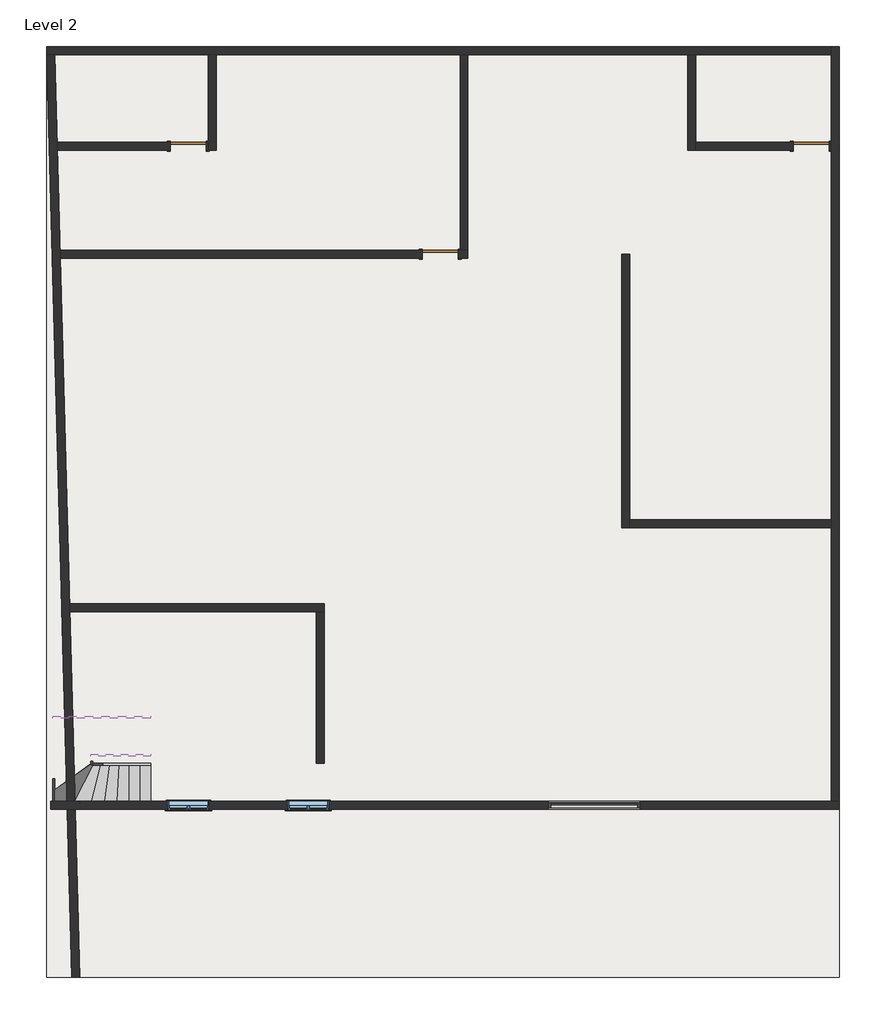
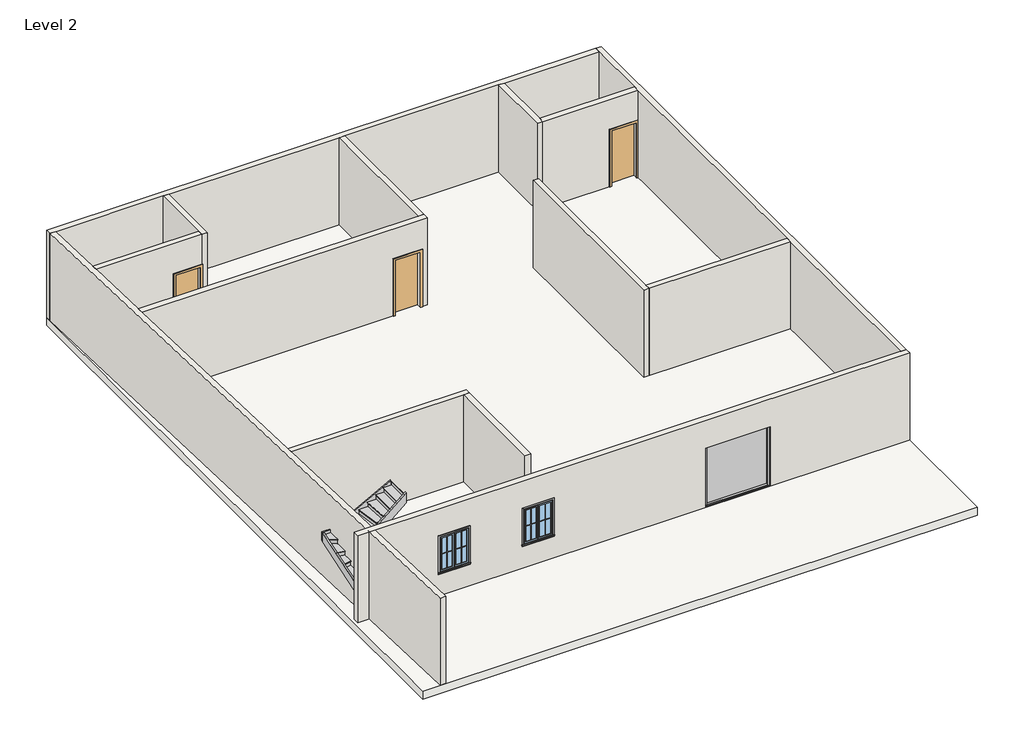
# One storey, incomplete: 14 walls, 11 members, 8 proxies, 3 doors, 2 windows, 1 plate, 1 slab, 1 stair flight.
"""IFC4 building model written with IfcOpenShell, lengths in millimetres."""

from ifc_helpers import new_model, si_unit, frame, origin, place, context, project, spatial, polyline, outline, extrude, faceted_brep, transform, mapped, element, save
from components import muntin_pattern_2x2_muntin_pattern_2x2_88bf7f41, muntin_pattern_2x2_muntin_pattern_2x2_3dfd0a47, trim_window_exterior_flat_with_sill_4930676f, trim_window_interior_flat_picture_frame_dd064338, door_54dd4da4, door_719f80de, member_a78380a5, member_04cfd63f, system_panel_glazed_45dfe0f7, stair_flight_257b0c60, window_0de3df1e

model = new_model("IFC4")

# Units and contexts
model_context = context("Model", 3, world=origin())
ifc_project = project(units=[si_unit("LENGTHUNIT", "METRE", prefix="MILLI")], contexts=[model_context])

# Site, building, storey
site = spatial("IfcSite", under=ifc_project)
building = spatial("IfcBuilding", under=site)
storey = spatial("IfcBuildingStorey", under=building, Name="Level 2", Elevation=3352.8)

# Proxies
placement = place(None, origin())
muntin_pattern_2x2_muntin_pattern_2x2_shape = muntin_pattern_2x2_muntin_pattern_2x2_88bf7f41(model_context)
element("IfcBuildingElementProxy", 1, Name="Muntin Pattern_2x2 : Muntin Pattern_2x2", ObjectType="Muntin Pattern_2x2 : Muntin Pattern_2x2", at=placement, inside=storey, context=model_context, shape_type="MappedRepresentation", body=[
    mapped(muntin_pattern_2x2_muntin_pattern_2x2_shape, transform((-6487.8306824, -10314.185779, 4337.05), x_axis=(-1.0, 0.0, 0.0), y_axis=(0.0, -1.0, 0.0), z_axis=(0.0, 0.0, 1.0))),
])
element("IfcBuildingElementProxy", 2, Name="Muntin Pattern_2x2 : Muntin Pattern_2x2", ObjectType="Muntin Pattern_2x2 : Muntin Pattern_2x2", at=placement, inside=storey, context=model_context, shape_type="MappedRepresentation", body=[
    mapped(muntin_pattern_2x2_muntin_pattern_2x2_shape, transform((-3439.8306824, -10314.185779, 4337.05), x_axis=(-1.0, 0.0, 0.0), y_axis=(0.0, -1.0, 0.0), z_axis=(0.0, 0.0, 1.0))),
])
muntin_pattern_2x2_muntin_pattern_2x2_2_shape = muntin_pattern_2x2_muntin_pattern_2x2_3dfd0a47(model_context)
element("IfcBuildingElementProxy", 3, Name="Muntin Pattern_2x2 : Muntin Pattern_2x2", ObjectType="Muntin Pattern_2x2 : Muntin Pattern_2x2", at=placement, inside=storey, context=model_context, shape_type="MappedRepresentation", body=[
    mapped(muntin_pattern_2x2_muntin_pattern_2x2_2_shape, transform((-7005.3556824, -10314.185779, 4337.05), x_axis=(1.0, 0.0, 0.0), y_axis=(0.0, 1.0, 0.0), z_axis=(0.0, 0.0, 1.0))),
])
element("IfcBuildingElementProxy", 4, Name="Muntin Pattern_2x2 : Muntin Pattern_2x2", ObjectType="Muntin Pattern_2x2 : Muntin Pattern_2x2", at=placement, inside=storey, context=model_context, shape_type="MappedRepresentation", body=[
    mapped(muntin_pattern_2x2_muntin_pattern_2x2_2_shape, transform((-3957.3556824, -10314.185779, 4337.05), x_axis=(1.0, 0.0, 0.0), y_axis=(0.0, 1.0, 0.0), z_axis=(0.0, 0.0, 1.0))),
])
trim_window_exterior_flat_with_sill_shape = trim_window_exterior_flat_with_sill_4930676f(model_context)
element("IfcBuildingElementProxy", 5, Name="Trim-Window-Exterior-Flat : with Sill", ObjectType="Trim-Window-Exterior-Flat : with Sill", at=placement, inside=storey, context=model_context, shape_type="MappedRepresentation", body=[
    mapped(trim_window_exterior_flat_with_sill_shape, transform((-6746.5931824, -10323.710779, 5613.4), x_axis=(1.0, 0.0, 0.0), y_axis=(0.0, 0.0, 1.0), z_axis=(0.0, -1.0, 0.0))),
])
element("IfcBuildingElementProxy", 6, Name="Trim-Window-Exterior-Flat : with Sill", ObjectType="Trim-Window-Exterior-Flat : with Sill", at=placement, inside=storey, context=model_context, shape_type="MappedRepresentation", body=[
    mapped(trim_window_exterior_flat_with_sill_shape, transform((-3698.5931824, -10323.710779, 5613.4), x_axis=(1.0, 0.0, 0.0), y_axis=(0.0, 0.0, 1.0), z_axis=(0.0, -1.0, 0.0))),
])
trim_window_interior_flat_picture_frame_shape = trim_window_interior_flat_picture_frame_dd064338(model_context)
element("IfcBuildingElementProxy", 7, Name="Trim-Window-Interior-Flat : Picture Frame", ObjectType="Trim-Window-Interior-Flat : Picture Frame", at=placement, inside=storey, context=model_context, shape_type="MappedRepresentation", body=[
    mapped(trim_window_interior_flat_picture_frame_shape, transform((-6746.5931824, -10120.510779, 5613.4), x_axis=(-1.0, 0.0, 0.0), y_axis=(0.0, 0.0, 1.0), z_axis=(0.0, 1.0, 0.0))),
])
element("IfcBuildingElementProxy", 8, Name="Trim-Window-Interior-Flat : Picture Frame", ObjectType="Trim-Window-Interior-Flat : Picture Frame", at=placement, inside=storey, context=model_context, shape_type="MappedRepresentation", body=[
    mapped(trim_window_interior_flat_picture_frame_shape, transform((-3698.5931824, -10120.510779, 5613.4), x_axis=(-1.0, 0.0, 0.0), y_axis=(0.0, 0.0, 1.0), z_axis=(0.0, 1.0, 0.0))),
])

# Doors
door_shape = door_54dd4da4(model_context)
element("IfcDoor", 9, ObjectType="Single-Flush : 36\" x 84\"", at=placement, inside=storey, context=model_context, shape_type="MappedRepresentation", body=[
    mapped(door_shape, transform((-345.7931824, 3798.689221, 3352.8), x_axis=(1.0, 0.0, 0.0), y_axis=(0.0, 1.0, 0.0), z_axis=(0.0, 0.0, 1.0))),
])
element("IfcDoor", 10, ObjectType="Single-Flush : 36\" x 84\"", at=placement, inside=storey, context=model_context, shape_type="MappedRepresentation", body=[
    mapped(door_shape, transform((-6746.5931824, 6541.889221, 3352.8), x_axis=(1.0, 0.0, 0.0), y_axis=(0.0, 1.0, 0.0), z_axis=(0.0, 0.0, 1.0))),
])
door_2_shape = door_719f80de(model_context)
element("IfcDoor", 11, ObjectType="Single-Flush : 36\" x 84\"", at=placement, inside=storey, context=model_context, shape_type="MappedRepresentation", body=[
    mapped(door_2_shape, transform((9103.0068176, 6541.889221, 3352.8), x_axis=(-1.0, 0.0, 0.0), y_axis=(0.0, -1.0, 0.0), z_axis=(0.0, 0.0, 1.0))),
])

# Members
member_shape = member_a78380a5(model_context)
element("IfcMember", 12, ObjectType="Rectangular Mullion : 2.5\" x 5\" rectangular", at=placement, inside=storey, context=model_context, shape_type="MappedRepresentation", body=[
    mapped(member_shape, transform((4743.1377464, -10222.110779, 3352.8), x_axis=(1.0, 0.0, 0.0), y_axis=(0.0, -1.0, 0.0), z_axis=(0.0, 0.0, -1.0))),
])
member_2_shape = member_04cfd63f(model_context)
element("IfcMember", 13, ObjectType="Rectangular Mullion : 2.5\" x 5\" rectangular", at=placement, inside=storey, context=model_context, shape_type="MappedRepresentation", body=[
    mapped(member_2_shape, transform((2465.1919806, -10222.110779, 3352.8), x_axis=(0.0, 0.0, -1.0), y_axis=(0.0, -1.0, 0.0), z_axis=(-1.0, 0.0, 0.0))),
])
element("IfcMember", 14, ObjectType="Rectangular Mullion : 2.5\" x 5\" rectangular", at=placement, inside=storey, context=model_context, shape_type="MappedRepresentation", body=[
    mapped(member_shape, transform((2401.6919806, -10222.110779, 6096.0), x_axis=(-1.0, 0.0, 0.0), y_axis=(0.0, -1.0, 0.0), z_axis=(0.0, 0.0, 1.0))),
])
element("IfcMember", 15, ObjectType="Stringer - 2\" Width", at=placement, inside=storey, context=model_context, shape_type="SweptSolid", body=[
    extrude(outline(polyline([(3352.8, -7708.0614906), (3585.2562572, -7708.0614906), (4706.3069249, -9795.4786823), (4360.3321542, -9795.4786823), (3352.8, -7919.4350738), (3352.8, -7708.0614906)])), frame((0.0, -10171.310779, 0.0), z_axis=(0.0, 1.0, 0.0), x_axis=(0.0, 0.0, 1.0)), (0.0, 0.0, 1.0), 50.8),
])
element("IfcMember", 16, ObjectType="Stringer - 2\" Width", at=placement, inside=storey, context=model_context, shape_type="SweptSolid", body=[
    extrude(outline(polyline([(-9795.4786823, -10120.510779), (-9795.4786823, -10171.310779), (-10150.1931824, -10171.310779), (-10150.1931824, -10120.510779), (-9795.4786823, -10120.510779)])), frame((0.0, 0.0, 4360.3321542), z_axis=(0.0, 0.0, 1.0), x_axis=(1.0, 0.0, 0.0)), (0.0, 0.0, 1.0), 345.9747707),
])
element("IfcMember", 17, ObjectType="Stringer - 2\" Width", at=placement, inside=storey, context=model_context, shape_type="SweptSolid", body=[
    extrude(outline(polyline([(-10171.310779, 4401.5069249), (-10171.310779, 4689.3201671), (-8051.2752516, 5398.2282369), (-8012.310779, 5398.2282369), (-8012.310779, 5065.2826013), (-9997.3749587, 4401.5069249), (-10171.310779, 4401.5069249)])), frame((-10200.9931824, 0.0, 0.0), z_axis=(1.0, 0.0, 0.0), x_axis=(0.0, 1.0, 0.0)), (0.0, 0.0, 1.0), 50.8),
])
element("IfcMember", 18, ObjectType="Stringer - 2\" Width", at=placement, inside=storey, context=model_context, shape_type="SweptSolid", body=[
    extrude(outline(polyline([(-10200.9931824, -8012.310779), (-10200.9931824, -7961.510779), (-9795.4786823, -7961.510779), (-9795.4786823, -8012.310779), (-10200.9931824, -8012.310779)])), frame((0.0, 0.0, 5076.8393171), z_axis=(0.0, 0.0, 1.0), x_axis=(1.0, 0.0, 0.0)), (0.0, 0.0, 1.0), 321.3889199),
])
element("IfcMember", 19, ObjectType="Stringer - 2\" Width", at=placement, inside=storey, context=model_context, shape_type="SweptSolid", body=[
    extrude(outline(polyline([(5398.2282369, -9795.4786823), (5076.8393171, -9795.4786823), (6197.8899847, -7708.0614906), (6519.2789046, -7708.0614906), (5398.2282369, -9795.4786823)])), frame((0.0, -8012.310779, 0.0), z_axis=(0.0, 1.0, 0.0), x_axis=(0.0, 0.0, 1.0)), (0.0, 0.0, 1.0), 50.8),
])
element("IfcMember", 20, ObjectType="Stringer - 2\" Width", at=placement, inside=storey, context=model_context, shape_type="SweptSolid", body=[
    extrude(outline(polyline([(3352.8, -7708.0614906), (3530.7241916, -7708.0614906), (4785.6713283, -9184.9931824), (4385.6989166, -9184.9931824), (3352.8, -7969.3872818), (3352.8, -7708.0614906)])), frame((0.0, -9206.110779, 0.0), z_axis=(0.0, 1.0, 0.0), x_axis=(0.0, 0.0, 1.0)), (0.0, 0.0, 1.0), 50.8),
])
element("IfcMember", 21, ObjectType="Stringer - 2\" Width", at=placement, inside=storey, context=model_context, shape_type="SweptSolid", body=[
    extrude(outline(polyline([(-9206.110779, 4428.8636174), (-9206.110779, 4989.3940989), (-9001.0207186, 5354.3714311), (-8977.510779, 5354.3714311), (-8977.510779, 4774.0173278), (-9171.4614414, 4428.8636174), (-9206.110779, 4428.8636174)])), frame((-9235.7931824, 0.0, 0.0), z_axis=(1.0, 0.0, 0.0), x_axis=(0.0, 1.0, 0.0)), (0.0, 0.0, 1.0), 50.8),
])
element("IfcMember", 22, ObjectType="Stringer - 2\" Width", at=placement, inside=storey, context=model_context, shape_type="SweptSolid", body=[
    extrude(outline(polyline([(5354.3714311, -9235.7931824), (4954.3990193, -9235.7931824), (6252.5108568, -7708.0614906), (6652.4832686, -7708.0614906), (5354.3714311, -9235.7931824)])), frame((0.0, -8977.510779, 0.0), z_axis=(0.0, 1.0, 0.0), x_axis=(0.0, 0.0, 1.0)), (0.0, 0.0, 1.0), 50.8),
])

# Plate
system_panel_glazed_shape = system_panel_glazed_45dfe0f7(model_context)
element("IfcPlate", 23, ObjectType="System Panel : Glazed", at=placement, inside=storey, context=model_context, shape_type="MappedRepresentation", body=[
    mapped(system_panel_glazed_shape, transform((3572.4148635, -10222.110779, 3416.3), x_axis=(1.0, 0.0, 0.0), y_axis=(0.0, 1.0, 0.0), z_axis=(0.0, 0.0, 1.0))),
])

# Slab
element("IfcSlab", 24, ObjectType="Generic - 12\"", at=placement, inside=storey, context=model_context, shape_type="SweptSolid", body=[
    extrude(outline(polyline([(-10353.3931824, -14590.910779), (-10353.3931824, 9081.889221), (9814.2068176, 9081.889221), (9814.2068176, -14590.910779), (-10353.3931824, -14590.910779)])), frame((0.0, 0.0, 3048.0), z_axis=(0.0, 0.0, 1.0), x_axis=(1.0, 0.0, 0.0)), (0.0, 0.0, 1.0), 304.8),
])

# Stair flight
stair_flight_shape = stair_flight_257b0c60(model_context)
element("IfcStairFlight", 25, ObjectType="2\" Tread 1\" Nosing 1/4\" Riser", at=placement, inside=storey, context=model_context, shape_type="MappedRepresentation", body=[
    mapped(stair_flight_shape, transform((0.0, 0.0, 0.0), x_axis=(1.0, 0.0, 0.0), y_axis=(0.0, 1.0, 0.0), z_axis=(0.0, 0.0, 1.0))),
])

# Walls
element("IfcWall", 26, ObjectType="wall.1", at=placement, inside=storey, context=model_context, shape_type="Brep", body=[
    faceted_brep([(-10350.6937129, 8878.689221, 3352.8), (-10147.4200314, 8878.689221, 3352.8), (-6238.5931824, 8878.689221, 3352.8), (-6035.3931824, 8878.689221, 3352.8), (162.2068176, 8878.689221, 3352.8), (365.4068176, 8878.689221, 3352.8), (5953.4068176, 8878.689221, 3352.8), (6156.6068176, 8878.689221, 3352.8), (9611.0068176, 8878.689221, 3352.8), (9611.0068176, 8878.689221, 6705.6), (6156.6068176, 8878.689221, 6705.6), (5953.4068176, 8878.689221, 6705.6), (365.4068176, 8878.689221, 6705.6), (162.2068176, 8878.689221, 6705.6), (-6035.3931824, 8878.689221, 6705.6), (-6238.5931824, 8878.689221, 6705.6), (-10147.4200314, 8878.689221, 6705.6), (-10350.6937129, 8878.689221, 6705.6), (-10356.1663335, 9081.889221, 3352.8), (-10356.1663335, 9081.889221, 6705.6), (9611.0068176, 9081.889221, 6705.6), (9611.0068176, 9081.889221, 3352.8)], [[[0, 1, 2, 3, 4, 5, 6, 7, 8, 9, 10, 11, 12, 13, 14, 15, 16, 17]], [[18, 19, 20, 21]], [[8, 7, 6, 5, 4, 3, 2, 1, 0, 18, 21]], [[17, 16, 15, 14, 13, 12, 11, 10, 9, 20, 19]], [[0, 17, 19, 18]], [[9, 8, 21, 20]]]),
])
element("IfcWall", 27, ObjectType="wall.1", at=placement, inside=storey, context=model_context, shape_type="Brep", body=[
    faceted_brep([(-9515.2300098, -14594.7106175, 3352.8), (-9765.7047419, -5294.510779, 3352.8), (-9771.1773626, -5091.310779, 3352.8), (-10007.8682051, 3697.089221, 3352.8), (-10013.3408258, 3900.289221, 3352.8), (-10081.7485837, 6440.289221, 3352.8), (-10087.2212044, 6643.489221, 3352.8), (-10147.4200314, 8878.689221, 3352.8), (-10147.4200314, 8878.689221, 6705.6), (-10087.2212044, 6643.489221, 6705.6), (-10081.7485837, 6440.289221, 6705.6), (-10013.3408258, 3900.289221, 6705.6), (-10007.8682051, 3697.089221, 6705.6), (-9771.1773626, -5091.310779, 6705.6), (-9765.7047419, -5294.510779, 6705.6), (-9515.2300098, -14594.7106175, 6705.6), (-9718.3563551, -14600.1812545, 3352.8), (-9718.3563551, -14600.1812545, 6705.6), (-10350.6937129, 8878.689221, 6705.6), (-10350.6937129, 8878.689221, 3352.8)], [[[0, 1, 2, 3, 4, 5, 6, 7, 8, 9, 10, 11, 12, 13, 14, 15]], [[16, 17, 18, 19]], [[7, 6, 5, 4, 3, 2, 1, 0, 16, 19]], [[15, 14, 13, 12, 11, 10, 9, 8, 18, 17]], [[0, 15, 17, 16]], [[8, 7, 19, 18]]]),
])
element("IfcWall", 28, ObjectType="wall.1", at=placement, inside=storey, context=model_context, shape_type="Brep", body=[
    faceted_brep([(9814.2068176, -10120.510779, 3352.8), (9611.0068176, -10120.510779, 3352.8), (-10251.7931824, -10120.510779, 3352.8), (-10251.7931824, -10120.510779, 6705.6), (9611.0068176, -10120.510779, 6705.6), (9814.2068176, -10120.510779, 6705.6), (4743.1377464, -10120.510779, 5638.8), (2401.6919806, -10120.510779, 5638.8), (2401.6919806, -10120.510779, 3375.5572706), (4743.1377464, -10120.510779, 3375.5572706), (-7267.2931824, -10120.510779, 5613.4), (-7267.2931824, -10120.510779, 4267.2), (-6225.8931824, -10120.510779, 4267.2), (-6225.8931824, -10120.510779, 5613.4), (-4219.2931824, -10120.510779, 5613.4), (-4219.2931824, -10120.510779, 4267.2), (-3177.8931824, -10120.510779, 4267.2), (-3177.8931824, -10120.510779, 5613.4), (-10251.7931824, -10323.710779, 3352.8), (9814.2068176, -10323.710779, 3352.8), (9814.2068176, -10323.710779, 6705.6), (-10251.7931824, -10323.710779, 6705.6), (2401.6919806, -10323.710779, 5638.8), (4743.1377464, -10323.710779, 5638.8), (4743.1377464, -10323.710779, 3375.5572706), (2401.6919806, -10323.710779, 3375.5572706), (-7267.2931824, -10323.710779, 5613.4), (-6225.8931824, -10323.710779, 5613.4), (-6225.8931824, -10323.710779, 4267.2), (-7267.2931824, -10323.710779, 4267.2), (-4219.2931824, -10323.710779, 5613.4), (-3177.8931824, -10323.710779, 5613.4), (-3177.8931824, -10323.710779, 4267.2), (-4219.2931824, -10323.710779, 4267.2)], [[[0, 1, 2, 3, 4, 5], [6, 7, 8, 9], [10, 11, 12, 13], [14, 15, 16, 17]], [[18, 19, 20, 21], [22, 23, 24, 25], [26, 27, 28, 29], [30, 31, 32, 33]], [[2, 1, 0, 19, 18]], [[3, 2, 18, 21]], [[5, 4, 3, 21, 20]], [[0, 5, 20, 19]], [[6, 23, 22, 7]], [[8, 25, 24, 9]], [[23, 6, 9, 24]], [[7, 22, 25, 8]], [[11, 10, 26, 29]], [[12, 11, 29, 28]], [[13, 12, 28, 27]], [[10, 13, 27, 26]], [[15, 14, 30, 33]], [[16, 15, 33, 32]], [[17, 16, 32, 31]], [[14, 17, 31, 30]]]),
])
element("IfcWall", 29, ObjectType="wall.1", at=placement, inside=storey, context=model_context, shape_type="Brep", body=[
    faceted_brep([(9611.0068176, 9081.889221, 3352.8), (9611.0068176, 8878.689221, 3352.8), (9611.0068176, 6643.489221, 3352.8), (9611.0068176, 6440.289221, 3352.8), (9611.0068176, -2957.710779, 3352.8), (9611.0068176, -3160.910779, 3352.8), (9611.0068176, -10120.510779, 3352.8), (9611.0068176, -10120.510779, 6705.6), (9611.0068176, -3160.910779, 6705.6), (9611.0068176, -2957.710779, 6705.6), (9611.0068176, 6440.289221, 6705.6), (9611.0068176, 6643.489221, 6705.6), (9611.0068176, 8878.689221, 6705.6), (9611.0068176, 9081.889221, 6705.6), (9814.2068176, 9081.889221, 3352.8), (9814.2068176, 9081.889221, 6705.6), (9814.2068176, -10120.510779, 6705.6), (9814.2068176, -10120.510779, 3352.8)], [[[0, 1, 2, 3, 4, 5, 6, 7, 8, 9, 10, 11, 12, 13]], [[14, 15, 16, 17]], [[6, 5, 4, 3, 2, 1, 0, 14, 17]], [[13, 12, 11, 10, 9, 8, 7, 16, 15]], [[0, 13, 15, 14]], [[7, 6, 17, 16]]]),
])
element("IfcWall", 30, ObjectType="wall.1", at=placement, inside=storey, context=model_context, shape_type="SweptSolid", body=[
    extrude(outline(polyline([(162.2068176, 3900.289221), (162.2068176, 8878.689221), (365.4068176, 8878.689221), (365.4068176, 3900.289221), (162.2068176, 3900.289221)])), frame((0.0, 0.0, 3352.8), z_axis=(0.0, 0.0, 1.0), x_axis=(1.0, 0.0, 0.0)), (0.0, 0.0, 1.0), 3352.8),
])
element("IfcWall", 31, ObjectType="wall.1", at=placement, inside=storey, context=model_context, shape_type="Brep", body=[
    faceted_brep([(365.4068176, 3900.289221, 3352.8), (162.2068176, 3900.289221, 3352.8), (111.4068176, 3900.289221, 3352.8), (111.4068176, 3900.289221, 5486.4), (-802.9931824, 3900.289221, 5486.4), (-802.9931824, 3900.289221, 3352.8), (-10013.3408258, 3900.289221, 3352.8), (-10013.3408258, 3900.289221, 6705.6), (162.2068176, 3900.289221, 6705.6), (365.4068176, 3900.289221, 6705.6), (111.4068176, 3697.089221, 5486.4), (111.4068176, 3697.089221, 3352.8), (365.4068176, 3697.089221, 3352.8), (365.4068176, 3697.089221, 6705.6), (-10007.8682051, 3697.089221, 6705.6), (-10007.8682051, 3697.089221, 3352.8), (-802.9931824, 3697.089221, 3352.8), (-802.9931824, 3697.089221, 5486.4)], [[[0, 1, 2, 3, 4, 5, 6, 7, 8, 9]], [[10, 11, 12, 13, 14, 15, 16, 17]], [[16, 15, 6, 5]], [[12, 11, 2, 1, 0]], [[9, 8, 7, 14, 13]], [[7, 6, 15, 14]], [[0, 9, 13, 12]], [[3, 2, 11, 10]], [[4, 3, 10, 17]], [[5, 4, 17, 16]]]),
])
element("IfcWall", 32, ObjectType="wall.1", at=placement, inside=storey, context=model_context, shape_type="Brep", body=[
    faceted_brep([(-6238.5931824, 8878.689221, 3352.8), (-6238.5931824, 6643.489221, 3352.8), (-6238.5931824, 6440.289221, 3352.8), (-6238.5931824, 6440.289221, 6705.6), (-6238.5931824, 6643.489221, 6705.6), (-6238.5931824, 8878.689221, 6705.6), (-6035.3931824, 8878.689221, 3352.8), (-6035.3931824, 8878.689221, 6705.6), (-6035.3931824, 6440.289221, 6705.6), (-6035.3931824, 6440.289221, 3352.8)], [[[0, 1, 2, 3, 4, 5]], [[6, 7, 8, 9]], [[2, 1, 0, 6, 9]], [[5, 4, 3, 8, 7]], [[0, 5, 7, 6]], [[3, 2, 9, 8]]]),
])
element("IfcWall", 33, ObjectType="wall.1", at=placement, inside=storey, context=model_context, shape_type="Brep", body=[
    faceted_brep([(-6238.5931824, 6643.489221, 3352.8), (-6289.3931824, 6643.489221, 3352.8), (-6289.3931824, 6643.489221, 5486.4), (-7203.7931824, 6643.489221, 5486.4), (-7203.7931824, 6643.489221, 3352.8), (-10087.2212044, 6643.489221, 3352.8), (-10087.2212044, 6643.489221, 6705.6), (-6238.5931824, 6643.489221, 6705.6), (-6289.3931824, 6440.289221, 5486.4), (-6289.3931824, 6440.289221, 3352.8), (-6238.5931824, 6440.289221, 3352.8), (-6238.5931824, 6440.289221, 6705.6), (-10081.7485837, 6440.289221, 6705.6), (-10081.7485837, 6440.289221, 3352.8), (-7203.7931824, 6440.289221, 3352.8), (-7203.7931824, 6440.289221, 5486.4)], [[[0, 1, 2, 3, 4, 5, 6, 7]], [[8, 9, 10, 11, 12, 13, 14, 15]], [[14, 13, 5, 4]], [[10, 9, 1, 0]], [[7, 6, 12, 11]], [[0, 7, 11, 10]], [[6, 5, 13, 12]], [[2, 1, 9, 8]], [[3, 2, 8, 15]], [[4, 3, 15, 14]]]),
])
element("IfcWall", 34, ObjectType="wall.1", at=placement, inside=storey, context=model_context, shape_type="Brep", body=[
    faceted_brep([(5953.4068176, 8878.689221, 3352.8), (5953.4068176, 6440.289221, 3352.8), (5953.4068176, 6440.289221, 6705.6), (5953.4068176, 8878.689221, 6705.6), (6156.6068176, 8878.689221, 3352.8), (6156.6068176, 8878.689221, 6705.6), (6156.6068176, 6643.489221, 6705.6), (6156.6068176, 6440.289221, 6705.6), (6156.6068176, 6440.289221, 3352.8), (6156.6068176, 6643.489221, 3352.8)], [[[0, 1, 2, 3]], [[4, 5, 6, 7, 8, 9]], [[1, 0, 4, 9, 8]], [[3, 2, 7, 6, 5]], [[0, 3, 5, 4]], [[2, 1, 8, 7]]]),
])
element("IfcWall", 35, ObjectType="wall.1", at=placement, inside=storey, context=model_context, shape_type="SweptSolid", body=[
    extrude(outline(polyline([(3352.8, 6156.6068176), (3352.8, 8645.8068176), (5486.4, 8645.8068176), (5486.4, 9560.2068176), (3352.8, 9560.2068176), (3352.8, 9611.0068176), (6705.6, 9611.0068176), (6705.6, 6156.6068176), (3352.8, 6156.6068176)])), frame((0.0, 6440.289221, 0.0), z_axis=(0.0, 1.0, 0.0), x_axis=(0.0, 0.0, 1.0)), (0.0, 0.0, 1.0), 203.2),
])
element("IfcWall", 36, ObjectType="wall.1", at=placement, inside=storey, context=model_context, shape_type="Brep", body=[
    faceted_brep([(4277.0068176, 3798.689221, 3352.8), (4277.0068176, -3160.910779, 3352.8), (4277.0068176, -3160.910779, 6705.6), (4277.0068176, 3798.689221, 6705.6), (4480.2068176, 3798.689221, 3352.8), (4480.2068176, 3798.689221, 6705.6), (4480.2068176, -2957.710779, 6705.6), (4480.2068176, -3160.910779, 6705.6), (4480.2068176, -3160.910779, 3352.8), (4480.2068176, -2957.710779, 3352.8)], [[[0, 1, 2, 3]], [[4, 5, 6, 7, 8, 9]], [[1, 0, 4, 9, 8]], [[3, 2, 7, 6, 5]], [[0, 3, 5, 4]], [[2, 1, 8, 7]]]),
])
element("IfcWall", 37, ObjectType="wall.1", at=placement, inside=storey, context=model_context, shape_type="SweptSolid", body=[
    extrude(outline(polyline([(9611.0068176, -3160.910779), (4480.2068176, -3160.910779), (4480.2068176, -2957.710779), (9611.0068176, -2957.710779), (9611.0068176, -3160.910779)])), frame((0.0, 0.0, 3352.8), z_axis=(0.0, 0.0, 1.0), x_axis=(1.0, 0.0, 0.0)), (0.0, 0.0, 1.0), 3352.8),
])
element("IfcWall", 38, ObjectType="wall.1", at=placement, inside=storey, context=model_context, shape_type="Brep", body=[
    faceted_brep([(-9765.7047419, -5294.510779, 3352.8), (-3495.3931824, -5294.510779, 3352.8), (-3292.1931824, -5294.510779, 3352.8), (-3292.1931824, -5294.510779, 6705.6), (-3495.3931824, -5294.510779, 6705.6), (-9765.7047419, -5294.510779, 6705.6), (-9771.1773626, -5091.310779, 3352.8), (-9771.1773626, -5091.310779, 6705.6), (-3292.1931824, -5091.310779, 6705.6), (-3292.1931824, -5091.310779, 3352.8)], [[[0, 1, 2, 3, 4, 5]], [[6, 7, 8, 9]], [[2, 1, 0, 6, 9]], [[5, 4, 3, 8, 7]], [[0, 5, 7, 6]], [[3, 2, 9, 8]]]),
])
element("IfcWall", 39, ObjectType="wall.1", at=placement, inside=storey, context=model_context, shape_type="SweptSolid", body=[
    extrude(outline(polyline([(-3495.3931824, -9155.310779), (-3495.3931824, -5294.510779), (-3292.1931824, -5294.510779), (-3292.1931824, -9155.310779), (-3495.3931824, -9155.310779)])), frame((0.0, 0.0, 3352.8), z_axis=(0.0, 0.0, 1.0), x_axis=(1.0, 0.0, 0.0)), (0.0, 0.0, 1.0), 3352.8),
])

# Windows
window_shape = window_0de3df1e(model_context)
element("IfcWindow", 40, ObjectType="Window-Casement-Double : 41\" x 53\"", at=placement, inside=storey, context=model_context, shape_type="MappedRepresentation", body=[
    mapped(window_shape, transform((-6746.5931824, -10222.110779, 3352.8), x_axis=(-1.0, 0.0, 0.0), y_axis=(0.0, -1.0, 0.0), z_axis=(0.0, 0.0, 1.0))),
])
element("IfcWindow", 41, ObjectType="Window-Casement-Double : 41\" x 53\"", at=placement, inside=storey, context=model_context, shape_type="MappedRepresentation", body=[
    mapped(window_shape, transform((-3698.5931824, -10222.110779, 3352.8), x_axis=(-1.0, 0.0, 0.0), y_axis=(0.0, -1.0, 0.0), z_axis=(0.0, 0.0, 1.0))),
])

save(model, "model.ifc")

# Revit data of these elements
# Type "Muntin Pattern_2x2 : Muntin Pattern_2x2"
#   Width [instance default] = 4' - 0"
#   Thickness = 0' - 0 1/2"
#   Height [instance default] = 4' - 0"
#   Distance = 0' - 0 3/4"
#   Interior Material [instance default] = none
#   Exterior Material [instance default] = none
#   Default Elevation = 0
# Type "Trim-Window-Exterior-Flat : with Sill"
#   Trim Width = 0' - 2 1/4"
#   Trim Thickness_Picture Frame = 0' - 1 1/4"
#   Trim Thickness_with Sill = 0' - 0 3/4"
#   Sill Thickness = 0' - 1 1/4"
#   Opening Width [instance default] = 2' - 0"
#   Opening Height [instance default] = 3' - 0"
#   Default Elevation = 4' - 0"
#   Sill = yes
#   Picture Frame = no
#   Trim Material [instance default] = none
# Type "Trim-Window-Interior-Flat : Picture Frame"
#   Trim Thickness_Picture Frame = 0' - 1 1/4"
#   Trim Width = 0' - 2 1/4"
#   Trim Thickness_with Sill = 0' - 0 3/4"
#   Sill Thickness = 0' - 1 1/4"
#   Opening Width [instance default] = 2' - 0"
#   Opening Height [instance default] = 3' - 0"
#   Default Elevation = 4' - 0"
#   Sill = no
#   Picture Frame = yes
#   Trim Material [instance default] = none
# Type "Single-Flush : 36\" x 84\""
#   Type Mark = "1"
#   Construction Type Id = "MDOOR"
#   Assembly Code = "C1020"
#   Analytic Construction = "Metal"
#   Thickness = 0' - 2"
#   Heat Transfer Coefficient (U) = 0.651978 BTU/(h·ft²·°F)
#   Height = 7' - 0"
#   Trim Projection Ext = 0' - 1"
#   Trim Projection Int = 0' - 1"
#   Trim Width = 0' - 3"
#   Width = 3' - 0"
#   Define Thermal Properties by = 1
#   Define Thermal Properties by = 1
#   Door Material = Door - Panel
#   Frame Material = Door - Frame
#   Visual Light Transmittance = 0
#   Solar Heat Gain Coefficient = 0
#   Function = (empty or 0)
#   Wall Closure = (empty or 0)
# Type "Rectangular Mullion : 2.5\" x 5\" rectangular"
#   built-in parameter 1007304 = 0.416667 (stored number, unit not read)
#   built-in parameter 1007301 = 0.104167 (stored number, unit not read)
#   built-in parameter 1007300 = 0.104167 (stored number, unit not read)
# Type "System Panel : Glazed"
#   Construction Type Id = "GSP4R"
#   Analytic Construction = "1/8 in Pilkington single glazing"
#   Visual Light Transmittance = 0.9
#   Solar Heat Gain Coefficient = 0.86
#   Heat Transfer Coefficient (U) = 1.18115 BTU/(h·ft²·°F)
#   Define Thermal Properties by = 1
# Type "Generic - 12\""
#   Assembly Code = "B1010"
#   Function = 0
#   Layers, outside or top first: 1' - 0" no material (function 1)
# Type "wall.1"
#   Assembly Code = "B2010"
#   Layers, outside or top first: 0' - 8" no material (function 1)
# Type "Window-Casement-Double : 41\" x 53\""
#   Type Mark = "15"
#   Fire Rating = "0.5h"
#   Assembly Code = "B2020100"
#   Analytic Construction = "Double glazing - domestic"
#   Frame Extension [instance default] = 0' - 0 1/4"
#   Window Inset [instance default] = 0' - 0"
#   Wall Thickness [instance default] = 0' - 6"
#   Interior Wall Closure [instance default] = 0' - 2 1/4"
#   Half Width = 1' - 8 1/2"
#   Visual Light Transmittance = 0.81
#   Thermal Resistance (R) = 1.8146 (h·ft²·°F)/BTU
#   Solar Heat Gain Coefficient = 0.76
#   Rough Width = 3' - 5 1/2"
#   Rough Height = 4' - 5 1/2"
#   Height = 4' - 5"
#   Heat Transfer Coefficient (U) = 0.5511 BTU/(h·ft²·°F)
#   Exterior Wall Closure [instance default] = 0' - 1 1/4"
#   Extension Jamb [instance default] = 0' - 2 1/4"
#   Default Sill Height = 3' - 0"
#   Width = 3' - 5"
#   Define Thermal Properties by = 0
#   Muntin Visibility = yes
#   Interior Trim Visibility [instance default] = yes
#   Exterior Trim Visibility [instance default] = yes
#   Extension Jamb Visibility [instance default] = yes
#   Interior Trim Material = Wood - Stained
#   Muntin Pattern = Muntin Pattern_2x2 : Muntin Pattern_2x2
#   Interior Trim = Trim-Window-Interior-Flat : Picture Frame
#   Interior Frame Material = Wood - Stained
#   Glass Panel Material = Glass
#   Exterior Trim Material = Clad - White
#   Exterior Trim = Trim-Window-Exterior-Flat : with Sill
#   Exterior Frame Material = Clad - White
#   Wall Closure = (empty or 0)
# Elements 1, 2, 3, 4 (IfcBuildingElementProxy, "Muntin Pattern_2x2 : Muntin Pattern_2x2")
#   Width = 1' - 3 1/8"
#   Height = 3' - 11 1/2"
#   Interior Material = Wood - Stained
#   Exterior Material = Clad - White
#   Phase Created = New Construction
#   Materials on its faces: "Clad - White", "Wood - Stained"
# Elements 5, 6 (IfcBuildingElementProxy, "Trim-Window-Exterior-Flat : with Sill")
#   Opening Width = 3' - 5"
#   Opening Height = 4' - 5"
#   Trim Material = Clad - White
#   Phase Created = New Construction
#   Materials on its faces: "Clad - White"
# Elements 7, 8 (IfcBuildingElementProxy, "Trim-Window-Interior-Flat : Picture Frame")
#   Opening Width = 3' - 5"
#   Opening Height = 4' - 5"
#   Trim Material = Wood - Stained
#   Phase Created = New Construction
#   Materials on its faces: "Wood - Stained"
# Elements 9, 10, 11 (IfcDoor, "Single-Flush : 36\" x 84\"")
#   Phase Created = New Construction
#   Materials on its faces: "Door - Frame", "Door - Panel"
# Elements 12, 13, 14 (IfcMember, "Rectangular Mullion : 2.5\" x 5\" rectangular")
#   Phase Created = New Construction
#   Materials on its faces: "Aluminum"
# Elements 15, 16, 17, 18, 19, 20, 21, 22 (IfcMember, "Stringer - 2\" Width")
#   Phase Created = New Construction
# Element 23 (IfcPlate, "System Panel : Glazed")
#   Phase Created = New Construction
#   Materials on its faces: "Glass"
# Element 24 (IfcSlab, "Generic - 12\"")
#   built-in parameter 1001955 = -1.5708 (stored number, unit not read)
#   Height Offset From Level = 0' - 0"
#   Phase Created = New Construction
#   Materials on its faces: "Default Floor", "GHT", "RG"
# Element 25 (IfcStairFlight, "2\" Tread 1\" Nosing 1/4\" Riser")
#   Phase Created = New Construction
# Elements 26, 27, 28, 29 (IfcWall, "wall.1")
#   Top Offset = 0' - 0"
#   Base Offset = 0' - 0"
#   Unconnected Height = 11' - 0"
#   wall height = 11' - 0"
#   Phase Created = New Construction
#   Base Constraint = Level 2
#   Materials on its faces: "Default Wall", "GHT"
# Elements 30, 31, 32, 33, 34, 35, 36, 37, 39 (IfcWall, "wall.1")
#   Top Offset = 0' - 0"
#   Base Offset = 0' - 0"
#   Unconnected Height = 11' - 0"
#   wall height = 11' - 0"
#   Phase Created = New Construction
#   Base Constraint = Level 2
#   Materials on its faces: "Default Wall"
# Element 38 (IfcWall, "wall.1")
#   Top Offset = 0' - 0"
#   Base Offset = 0' - 0"
#   Unconnected Height = 11' - 0"
#   wall height = 11' - 0"
#   Phase Created = New Construction
#   Base Constraint = Level 2
#   Materials on its faces: "Default Wall", "Wood - Stained"
# Element 40 (IfcWindow, "Window-Casement-Double : 41\" x 53\"")
#   Mark = "1"
#   Window Inset = 0' - 0"
#   Interior Wall Closure = 0' - 2 1/4"
#   Frame Extension = 0' - 0 1/4"
#   Exterior Wall Closure = 0' - 1 1/4"
#   Interior Trim Visibility = yes
#   Exterior Trim Visibility = yes
#   Phase Created = New Construction
#   Materials on its faces: "Wood - Stained", "Glass", "Clad - White"
# Element 41 (IfcWindow, "Window-Casement-Double : 41\" x 53\"")
#   Mark = "2"
#   Window Inset = 0' - 0"
#   Interior Wall Closure = 0' - 2 1/4"
#   Frame Extension = 0' - 0 1/4"
#   Exterior Wall Closure = 0' - 1 1/4"
#   Interior Trim Visibility = yes
#   Exterior Trim Visibility = yes
#   Phase Created = New Construction
#   Materials on its faces: "Wood - Stained", "Glass", "Clad - White"
# Materials
#   "Door - Panel": class "Wood", colour RGB 210 159 95, transparency 0, Cost = 0
#   "Door - Frame": colour RGB 118 70 51, transparency 0, Cost = 0
#   "Wood - Stained": class "Wood", colour RGB 224 178 126, transparency 0, Cost = 0
#   "Glass": class "Glass", colour RGB 0 128 192, transparency 0.75, Description = "Soda Lime Glass", Cost = 0
#   "Clad - White": class "Wood", colour RGB 242 242 238, transparency 0, Cost = 0
#   "Aluminum": class "Metal", colour RGB 247 247 247, transparency 0, Description = "Aluminum 6061", Cost = 0
#   "Default Floor": colour RGB 128 128 128, transparency 0, Cost = 0
#   "GHT": class "Generic", colour RGB 120 120 120, transparency 0, Cost = 0
#   "RG": class "Generic", colour RGB 120 120 120, transparency 0, Cost = 0
#   "Default Wall": colour RGB 128 128 128, transparency 0, Cost = 0
